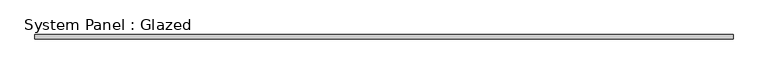
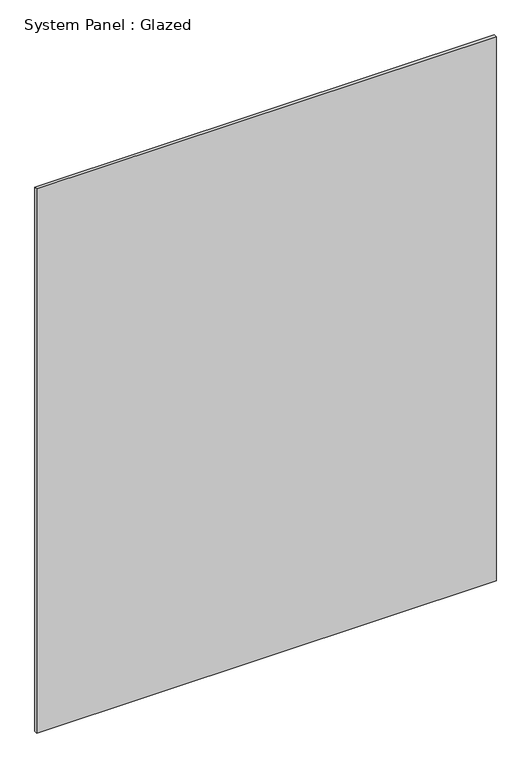
"""IFC4 building model written with IfcOpenShell, lengths in millimetres: plate geometry, System Panel : Glazed."""

from ifc_helpers import new_model, si_unit, origin, origin_with_axes, place, context, project, spatial, polyline, outline, extrude, source, transform, mapped, element, save


def system_panel_glazed_ccff25ac(model_context):
    return source(origin(), model_context, "Body", "SweptSolid", [
        extrude(outline(polyline([(2017.8542392, 19.05), (-2017.8542392, 19.05), (-2017.8542392, 44.45), (2017.8542392, 44.45), (2017.8542392, 19.05)])), origin_with_axes(), (0.0, 0.0, 1.0), 5054.6),
    ])


if __name__ == "__main__":
    model = new_model("IFC4")
    model_context = context("Model", 3, world=origin())
    ifc_project = project(units=[si_unit("LENGTHUNIT", "METRE", prefix="MILLI")], contexts=[model_context])
    site = spatial("IfcSite", under=ifc_project)
    building = spatial("IfcBuilding", under=site)
    placement = place(None, origin())
    system_panel_glazed_shape = system_panel_glazed_ccff25ac(model_context)
    element("IfcPlate", 1, ObjectType="System Panel : Glazed", at=placement, inside=building, context=model_context, shape_type="MappedRepresentation", body=[
        mapped(system_panel_glazed_shape, transform((0.0, 0.0, 0.0), x_axis=(1.0, 0.0, 0.0), y_axis=(0.0, 1.0, 0.0), z_axis=(0.0, 0.0, 1.0))),
    ])
    save(model, "model.ifc")

# Revit data of these elements
# Type "System Panel : Glazed"
#   Construction Type Id = "GSP4R"
#   Analytic Construction = "1/8 in Pilkington single glazing"
#   Visual Light Transmittance = 0.9
#   Solar Heat Gain Coefficient = 0.86
#   Heat Transfer Coefficient (U) = 1.18115 BTU/(h·ft²·°F)
# Element 1 (IfcPlate, "System Panel : Glazed")
#   Materials on its faces: "Glass"
# Materials
#   "Glass": class "Glass", colour RGB 0 128 192, transparency 0.75, Description = "Soda Lime Glass", Cost = 0
